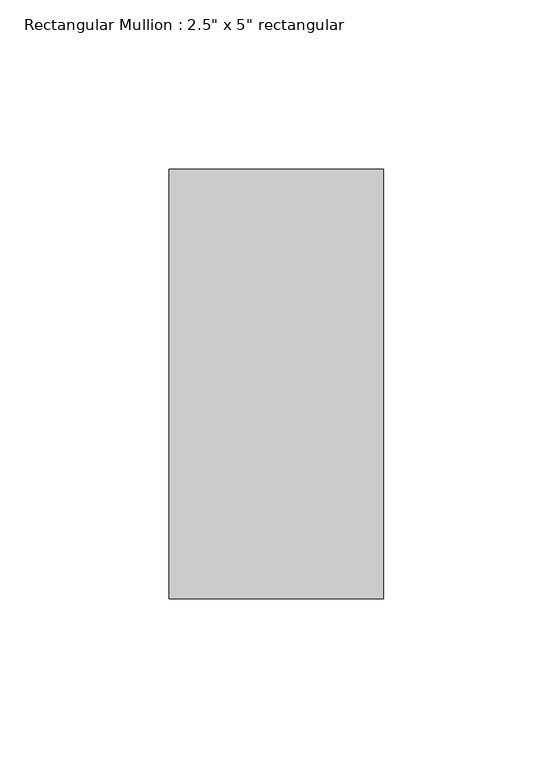
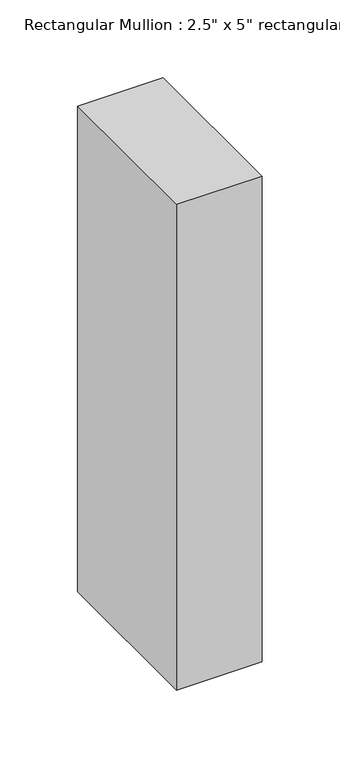
"""IFC4 building model written with IfcOpenShell, lengths in millimetres: member geometry."""

from ifc_helpers import new_model, si_unit, frame, origin, place, context, project, spatial, polyline, outline, extrude, source, transform, mapped, element, save


def member_03a502dc(model_context):
    return source(origin(), model_context, "Body", "SweptSolid", [
        extrude(outline(polyline([(31.75, 63.5), (31.75, -63.5), (-31.75, -63.5), (-31.75, 63.5), (31.75, 63.5)])), frame((0.0, 0.0, -381.0), z_axis=(0.0, 0.0, 1.0), x_axis=(1.0, 0.0, 0.0)), (0.0, 0.0, 1.0), 381.0),
    ])


if __name__ == "__main__":
    model = new_model("IFC4")
    model_context = context("Model", 3, world=origin())
    ifc_project = project(units=[si_unit("LENGTHUNIT", "METRE", prefix="MILLI")], contexts=[model_context])
    site = spatial("IfcSite", under=ifc_project)
    building = spatial("IfcBuilding", under=site)
    placement = place(None, origin())
    member_shape = member_03a502dc(model_context)
    element("IfcMember", 1, ObjectType="Rectangular Mullion : 2.5\" x 5\" rectangular", at=placement, inside=building, context=model_context, shape_type="MappedRepresentation", body=[
        mapped(member_shape, transform((0.0, 0.0, 0.0), x_axis=(1.0, 0.0, 0.0), y_axis=(0.0, 1.0, 0.0), z_axis=(0.0, 0.0, 1.0))),
    ])
    save(model, "model.ifc")

# Revit data of these elements
# Type "Rectangular Mullion : 2.5\" x 5\" rectangular"
#   built-in parameter 1007304 = 0.416667 (stored number, unit not read)
#   built-in parameter 1007301 = 0.104167 (stored number, unit not read)
#   built-in parameter 1007300 = 0.104167 (stored number, unit not read)
# Element 1 (IfcMember, "Rectangular Mullion : 2.5\" x 5\" rectangular")
#   Materials on its faces: "Aluminum"
# Materials
#   "Aluminum": class "Metal", colour RGB 247 247 247, transparency 0, Description = "Aluminum 6061", Cost = 0
